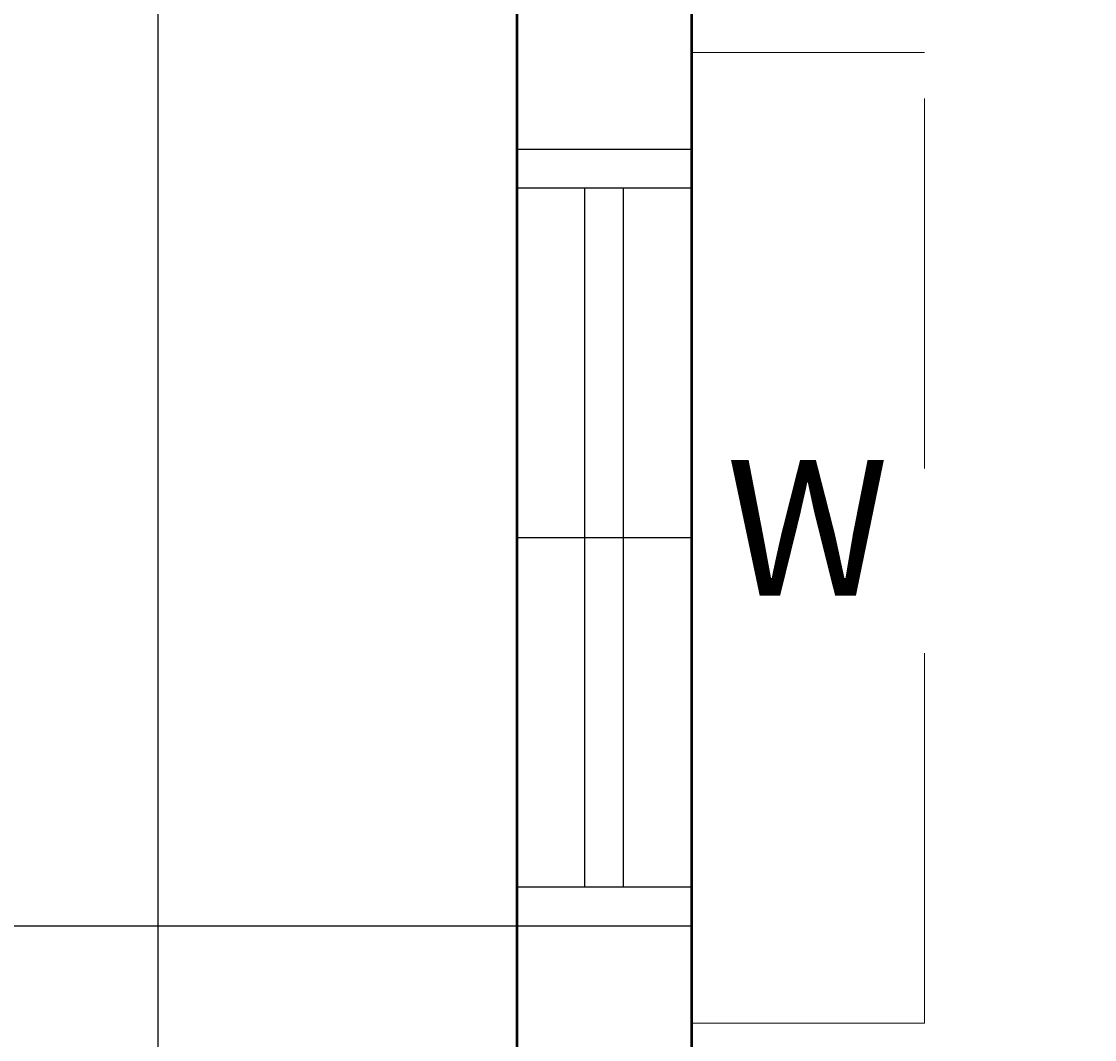
# Model space of a CAD drawing. Units: inches. Extents: x 37 to 824, y -700 to 234.
# Tile 72 of 77: x 394 to 449, y 107 to 160. Entities that reach past the tile are written whole.
import ezdxf

# ---------------------------------------------------------------- set-up
doc = ezdxf.new("R2010")
doc.units = ezdxf.units.IN
doc.header["$MEASUREMENT"] = 0
doc.linetypes.add('DASHED', pattern=[19.05, 12.7, -6.35])
for name, color, linetype, lineweight in [('A-ANNO-DIMS', 2, 'Continuous', 18), ('A-ANNO-TEXT', 7, 'Continuous', 18), ('A-GLAZ', 4, 'Continuous', 25), ('A-ROOF-OVHD', 1, 'DASHED', 18), ('A-WALL', 2, 'Continuous', 50)]:
    doc.layers.add(name, color=color, linetype=linetype, lineweight=lineweight)
doc.styles.get("Standard").update_dxf_attribs({"font": 'arial.ttf'})
doc.dimstyles.get("Standard").update_dxf_attribs({"dimtxt": 0.18, "dimasz": 0.18, "dimexe": 0.18, "dimexo": 0.0625, "dimgap": 0.09, "dimtad": 0, "dimtih": 1, "dimtoh": 1, "dimdec": 1, "dimzin": 0, "dimdsep": 46, "dimlunit": 4, "dimtxsty": 'Standard', "dimcen": 0.09, "dimadec": 0, "dimazin": 0, "dimtfac": 1, "dimtdec": 1, "dimtofl": 0, "dimtmove": 0, "dimatfit": 3, "dimfxl": 1, "dimtolj": 1, "dimtzin": 0, "dimarcsym": 0})

# ---------------------------------------------------------------- blocks, each defined once
blk = doc.blocks.new('WIN-900')
for p, q in [((0, 9), (0, 0)), ((2, 9), (2, 0)), ((20, 9), (20, 0)), ((38, 9), (38, 0)), ((40, 9), (40, 0)), ((38, 5.5), (2, 5.5)), ((38, 3.5), (2, 3.5))]:
    blk.add_line(p, q)
blk = doc.blocks.new('*D60')
at = {"layer": 'A-ANNO-DIMS', "color": 0, "lineweight": -2, "ltscale": 0.5, "transparency": 16777216}
for p, q in [((419.015, 113.09), (78.159, 113.09)), ((78.339, 112.91), (78.339, 98.772)), ((78.339, 84.27), (78.339, 98.409)), ((419.015, 84.09), (78.159, 84.09))]:
    blk.add_line(p, q, dxfattribs=at)
at = {"layer": 'A-ANNO-DIMS', "color": 0, "ltscale": 0.5, "transparency": 16777216}
for points in [[(78.309, 112.91), (78.369, 112.91), (78.339, 113.09)], [(78.309, 84.27), (78.369, 84.27), (78.339, 84.09)]]:
    blk.add_solid(points, dxfattribs=at)
at = {"layer": 'Defpoints', "color": 0, "ltscale": 0.5, "transparency": 16777216}
for p in [(78.339, 113.09), (419.077, 113.09), (419.077, 84.09)]:
    blk.add_point(p, dxfattribs=at)
at = {"layer": 'A-ANNO-DIMS', "color": 0, "ltscale": 0.5, "transparency": 16777216, "insert": (78.339, 98.59), "char_height": 0.18, "attachment_point": 5}
blk.add_mtext('\\A1;2\'-5"', dxfattribs=at)
blk = doc.blocks.new('*D64')
at = {"layer": 'A-ANNO-DIMS', "color": 0, "lineweight": -2, "ltscale": 0.5, "transparency": 16777216}
for p, q in [((428.14, 191.09), (513.773, 191.09)), ((513.593, 190.91), (513.593, -87.228)), ((513.593, -365.73), (513.593, -87.591)), ((428.14, -365.91), (513.773, -365.91))]:
    blk.add_line(p, q, dxfattribs=at)
at = {"layer": 'A-ANNO-DIMS', "color": 0, "ltscale": 0.5, "transparency": 16777216}
for points in [[(513.563, 190.91), (513.623, 190.91), (513.593, 191.09)], [(513.563, -365.73), (513.623, -365.73), (513.593, -365.91)]]:
    blk.add_solid(points, dxfattribs=at)
at = {"layer": 'Defpoints', "color": 0, "ltscale": 0.5, "transparency": 16777216}
for p in [(428.077, 191.09), (428.077, -365.91), (513.593, -365.91)]:
    blk.add_point(p, dxfattribs=at)
at = {"layer": 'A-ANNO-DIMS', "color": 0, "ltscale": 0.5, "transparency": 16777216, "insert": (513.593, -87.41), "char_height": 0.18, "attachment_point": 5}
blk.add_mtext('\\A1;46\'-5"', dxfattribs=at)
blk = doc.blocks.new('*D74')
at = {"layer": 'A-ANNO-DIMS', "color": 0, "lineweight": -2, "ltscale": 0.5, "transparency": 16777216}
for p, q in [((371.077, 84.153), (371.077, 234.17)), ((371.257, 233.99), (385.3, 233.99)), ((400.425, 233.99), (386.381, 233.99)), ((400.605, 84.153), (400.605, 234.17))]:
    blk.add_line(p, q, dxfattribs=at)
at = {"layer": 'A-ANNO-DIMS', "color": 0, "ltscale": 0.5, "transparency": 16777216}
for points in [[(371.257, 234.02), (371.257, 233.96), (371.077, 233.99)], [(400.425, 234.02), (400.425, 233.96), (400.605, 233.99)]]:
    blk.add_solid(points, dxfattribs=at)
at = {"layer": 'Defpoints', "color": 0, "ltscale": 0.5, "transparency": 16777216}
for p in [(400.605, 233.99), (371.077, 84.09), (400.605, 84.09)]:
    blk.add_point(p, dxfattribs=at)
at = {"layer": 'A-ANNO-DIMS', "color": 0, "ltscale": 0.5, "transparency": 16777216, "insert": (385.841, 233.99), "char_height": 0.18, "attachment_point": 5}
blk.add_mtext('\\A1;2\'-5 1/2"', dxfattribs=at)
blk = doc.blocks.new('*D75')
at = {"layer": 'A-ANNO-DIMS', "color": 0, "lineweight": -2, "ltscale": 0.5, "transparency": 16777216}
for p, q in [((400.605, 84.153), (400.605, 234.17)), ((400.785, 233.99), (409.31, 233.99)), ((418.897, 233.99), (410.371, 233.99)), ((419.077, 84.153), (419.077, 234.17))]:
    blk.add_line(p, q, dxfattribs=at)
at = {"layer": 'A-ANNO-DIMS', "color": 0, "ltscale": 0.5, "transparency": 16777216}
for points in [[(400.785, 234.02), (400.785, 233.96), (400.605, 233.99)], [(418.897, 234.02), (418.897, 233.96), (419.077, 233.99)]]:
    blk.add_solid(points, dxfattribs=at)
at = {"layer": 'Defpoints', "color": 0, "ltscale": 0.5, "transparency": 16777216}
for p in [(419.077, 233.99), (400.605, 84.09), (419.077, 84.09)]:
    blk.add_point(p, dxfattribs=at)
at = {"layer": 'A-ANNO-DIMS', "color": 0, "ltscale": 0.5, "transparency": 16777216, "insert": (409.841, 233.99), "char_height": 0.18, "attachment_point": 5}
blk.add_mtext('\\A1;1\'-6 1/2"', dxfattribs=at)
blk = doc.blocks.new('*D83')
at = {"layer": 'A-ANNO-DIMS', "color": 0, "lineweight": -2, "ltscale": 0.5, "transparency": 16777216}
for p, q in [((358.132, -206.847), (358.132, 234.17)), ((358.312, 233.99), (388.275, 233.99)), ((418.897, 233.99), (388.934, 233.99)), ((419.077, -206.847), (419.077, 234.17))]:
    blk.add_line(p, q, dxfattribs=at)
at = {"layer": 'A-ANNO-DIMS', "color": 0, "ltscale": 0.5, "transparency": 16777216}
for points in [[(358.312, 234.02), (358.312, 233.96), (358.132, 233.99)], [(418.897, 234.02), (418.897, 233.96), (419.077, 233.99)]]:
    blk.add_solid(points, dxfattribs=at)
at = {"layer": 'Defpoints', "color": 0, "ltscale": 0.5, "transparency": 16777216}
for p in [(419.077, 233.99), (358.132, -206.91), (419.077, -206.91)]:
    blk.add_point(p, dxfattribs=at)
at = {"layer": 'A-ANNO-DIMS', "color": 0, "ltscale": 0.5, "transparency": 16777216, "insert": (388.605, 233.99), "char_height": 0.18, "attachment_point": 5}
blk.add_mtext('\\A1;5\'-1"', dxfattribs=at)

msp = doc.modelspace()

# ---------------------------------------------------------------- linework, layer by layer
at = {"layer": 'A-ROOF-OVHD', "ltscale": 1.5}
for p, q in [((428.077, 153.09), (428.077, 158.09)), ((428.077, 158.09), (440.077, 158.09)), ((440.077, 108.09), (440.077, 158.09)), ((428.077, 113.09), (428.077, 108.09)), ((428.077, 108.09), (440.077, 108.09))]:
    msp.add_line(p, q, dxfattribs=at)
at = {"layer": 'A-WALL'}
for p, q in [((428.077, 191.09), (428.077, 75.09)), ((419.077, 182.09), (419.077, 84.09))]:
    msp.add_line(p, q, dxfattribs=at)

# ---------------------------------------------------------------- block references
at = {"layer": 'A-GLAZ', "rotation": 270.0000000000001}
msp.add_blockref('WIN-900', (419.077, 153.091), dxfattribs=at)

# ---------------------------------------------------------------- texts
at = {"layer": 'A-ANNO-TEXT'}
msp.add_text('W', height=7, dxfattribs=at).set_placement((429.865, 130.103))

# ---------------------------------------------------------------- dimensions: what is measured, and where the dimension line sits
at = {"layer": 'A-ANNO-DIMS', "ltscale": 0.5}
for base, p1, p2, picture, middle in [((419.077, 233.99), (358.132, -206.91), (419.077, -206.91), '*D83', (388.605, 233.99)), ((400.605, 233.99), (371.077, 84.09), (400.605, 84.09), '*D74', (385.841, 233.99)), ((419.077, 233.99), (400.605, 84.09), (419.077, 84.09), '*D75', (409.841, 233.99))]:
    dim = msp.add_linear_dim(base=base, p1=p1, p2=p2, dimstyle='Standard', override={"dimdec": 1, "dimlfac": 1, "dimrnd": 0, "dimzin": 1, "dimdsep": 46, "dimlunit": 4, "dimfrac": 2}, dxfattribs=at)
    dim.commit()
    dim.dimension.update_dxf_attribs({"geometry": picture, "text_midpoint": middle})
for base, p1, p2, picture, middle in [((513.593, -365.91), (428.077, 191.09), (428.077, -365.91), '*D64', (513.593, -87.41)), ((78.339, 113.09), (419.077, 84.09), (419.077, 113.09), '*D60', (78.339, 98.59))]:
    dim = msp.add_linear_dim(base=base, p1=p1, p2=p2, angle=90, dimstyle='Standard', override={"dimdec": 1, "dimlfac": 1, "dimrnd": 0, "dimzin": 1, "dimdsep": 46, "dimlunit": 4, "dimfrac": 2}, dxfattribs=at)
    dim.commit()
    dim.dimension.update_dxf_attribs({"geometry": picture, "text_midpoint": middle})

doc.saveas('drawing.dxf')
